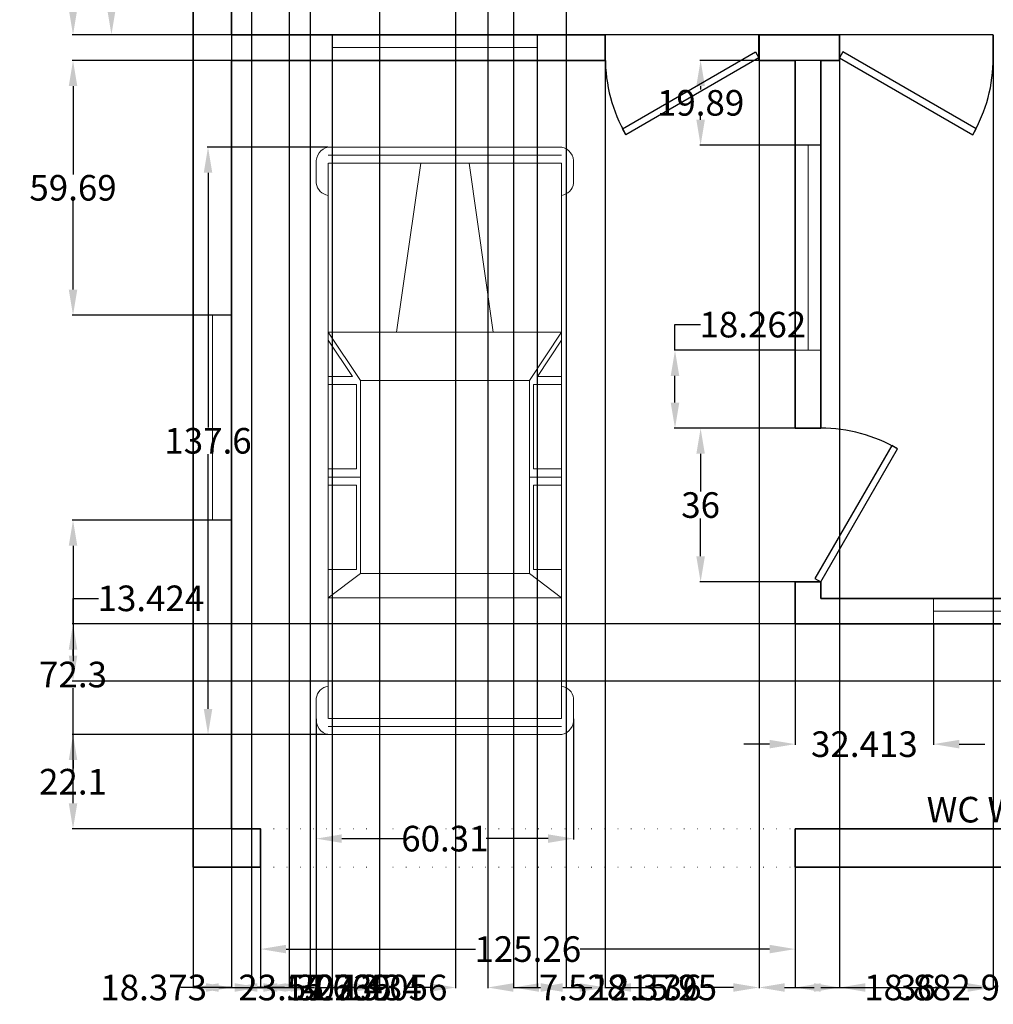
# Model space of a CAD drawing. Units: inches. Extents: x 351 to 774, y 111 to 703.
# Tile 1 of 6: x 380 to 608, y 111 to 342. Entities that reach past the tile are written whole.
import ezdxf

# ---------------------------------------------------------------- set-up
doc = ezdxf.new("R2010")
doc.units = ezdxf.units.IN
doc.header["$MEASUREMENT"] = 0
doc.linetypes.add('ACAD_ISO07W100', pattern=[3, 0, -3])
for name, color, linetype, lineweight in [('A-ANNO-DIMS', 2, 'Continuous', 18), ('A-DOOR', 3, 'Continuous', 25), ('A-EQPM-VEHC', 8, 'Continuous', 13), ('A-GLAZ', 4, 'Continuous', 18), ('A-WALL', 7, 'Continuous', 35), ('A-WALL-OVHD', 7, 'ACAD_ISO07W100', 18)]:
    doc.layers.add(name, color=color, linetype=linetype, lineweight=lineweight)
doc.styles.get("Standard").update_dxf_attribs({"font": 'arial.ttf'})
doc.dimstyles.get("Standard").update_dxf_attribs({"dimtxt": 6, "dimasz": 6, "dimexe": 0.18, "dimexo": 0.0625, "dimgap": 0.09, "dimtad": 0, "dimtih": 1, "dimtoh": 1, "dimdec": 0, "dimzin": 0, "dimdsep": 46, "dimlunit": 3, "dimtxsty": 'Standard', "dimcen": 0.09, "dimadec": 0, "dimazin": 0, "dimtfac": 1, "dimtdec": 0, "dimtofl": 0, "dimtmove": 0, "dimatfit": 3, "dimfxl": 1, "dimtolj": 1, "dimtzin": 0, "dimarcsym": 0})

# ---------------------------------------------------------------- blocks, each defined once
blk = doc.blocks.new('*U4')
for p, q in [((-40, 0), (-40, 6)), ((0, 0), (0, 6))]:
    blk.add_line(p, q)
blk.add_lwpolyline([(0, 0), (-34.64, -20), (-35.52, -18.48), (-0.88, 1.52)], close=True)
blk.add_arc((0, 0), 40, 180, 210)
blk = doc.blocks.new('*U5')
for p, q in [((0, 0), (0, 6)), ((40, 0), (40, 6))]:
    blk.add_line(p, q)
blk.add_lwpolyline([(0, 0), (34.64, -20), (35.52, -18.48), (0.88, 1.52)], close=True)
blk.add_arc((0, 0), 40, 330, 0)
blk = doc.blocks.new('*U6')
for p, q in [((0, 0), (0, -6)), ((-40, 0), (-40, -6))]:
    blk.add_line(p, q)
blk.add_lwpolyline([(0, 0), (-34.64, 20), (-35.52, 18.48), (-0.88, -1.52)], close=True)
blk.add_arc((0, 0), 40, 150, 180)
blk = doc.blocks.new('*U15')
for p, q in [((5.44, 42.31), (12.12, 42.31)), ((189.69, 42.31), (183.01, 42.31)), ((0.1, -0.41), (0.1, 38.35)), ((2.77, -0.41), (2.77, 38.31)), ((5.44, -0.41), (5.44, 38.24)), ((5.45, 38.31), (16.12, 38.31)), ((16.12, 38.31), (180.34, 38.31)), ((61.52, -0.41), (61.52, 38.31)), ((61.52, 38.31), (77.54, 27.62)), ((64.19, 38.31), (76.2, 30.29)), ((76.2, 30.29), (76.2, 38.31)), ((78.87, 38.31), (78.87, 28.96)), ((106.91, 28.96), (106.91, 38.31)), ((109.58, 27.62), (109.58, 38.31)), ((112.25, 38.31), (112.25, 28.96)), ((140.29, 28.96), (140.29, 38.31)), ((141.62, 27.62), (149.64, 38.31)), ((149.64, -0.41), (149.64, 38.31)), ((189.69, 38.31), (179.01, 38.31)), ((189.69, -0.41), (189.69, 38.24)), ((192.36, -0.41), (192.36, 38.31)), ((195.03, -0.41), (195.03, 38.35)), ((77.54, 27.62), (141.62, 27.62)), ((77.54, -0.41), (77.54, 27.62)), ((78.87, 28.96), (106.91, 28.96)), ((112.25, 28.96), (140.29, 28.96)), ((141.62, -0.41), (141.62, 27.62)), ((5.44, 7.6), (61.52, 15.61)), ((0.1, -0.42), (0.1, -39.18)), ((2.77, -0.41), (2.77, -39.13)), ((5.44, -0.42), (5.44, -39.07)), ((61.52, -0.41), (61.52, -39.13)), ((77.54, -0.41), (77.54, -28.45)), ((141.62, -0.41), (141.62, -28.45)), ((149.64, -0.41), (149.64, -39.13)), ((189.69, -0.42), (189.69, -39.07)), ((192.36, -0.41), (192.36, -39.13)), ((195.03, -0.42), (195.03, -39.18)), ((5.44, -8.42), (61.52, -16.43)), ((61.52, -39.13), (77.54, -28.45)), ((77.54, -28.45), (141.62, -28.45)), ((109.58, -28.45), (109.58, -39.13)), ((141.62, -28.45), (149.64, -39.13)), ((64.19, -39.13), (76.2, -31.12)), ((76.2, -31.12), (76.2, -39.13)), ((78.87, -39.13), (78.87, -29.79)), ((78.87, -29.79), (106.91, -29.79)), ((106.91, -29.79), (106.91, -39.13)), ((112.25, -29.79), (140.29, -29.79)), ((112.25, -39.13), (112.25, -29.79)), ((140.29, -29.79), (140.29, -39.13)), ((5.45, -39.13), (16.12, -39.13)), ((16.12, -39.13), (180.34, -39.13)), ((189.69, -39.13), (179.01, -39.13)), ((5.44, -43.14), (12.12, -43.14)), ((189.69, -43.14), (183.01, -43.14))]:
    blk.add_line(p, q)
for centre, radius, start, end in [((5.06, 37.26), 5.06, 85.6455, 168.0943), ((11.45, 37.64), 4.72, 8.1301, 81.87), ((183.68, 37.64), 4.72, 98.13, 171.8699), ((190.07, 37.26), 5.06, 11.9057, 94.3545), ((5.06, -38.09), 5.06, 191.9057, 274.3545), ((11.45, -38.46), 4.72, 278.13, 351.8699), ((183.68, -38.46), 4.72, 188.1301, 261.87), ((190.07, -38.09), 5.06, 265.6455, 348.0943)]:
    blk.add_arc(centre, radius, start, end)
blk = doc.blocks.new('WIN-48IN-6IN-WALL')
blk.add_line((3, 48), (3, 0))
blk.add_lwpolyline([(0, 48), (6, 48), (6, 0), (0, 0)], close=True)
blk = doc.blocks.new('WIN-48IN-9IN-WALL')
blk.add_line((4.5, 48), (4.5, 0))
blk.add_lwpolyline([(0, 0), (9, 0), (9, 48), (0, 48)], close=True)
blk = doc.blocks.new('*D26')
at = {"layer": 'A-ANNO-DIMS', "color": 0, "lineweight": -2, "transparency": 16777216}
for p, q in [((680.41, 152.3), (680.41, 156.92)), ((710.41, 152.3), (710.41, 156.92)), ((680.41, 156.74), (674.41, 156.74)), ((704.41, 156.74), (686.41, 156.74))]:
    blk.add_line(p, q, dxfattribs=at)
at = {"layer": 'A-ANNO-DIMS', "color": 0, "transparency": 16777216}
for points in [[(686.41, 157.74), (686.41, 155.74), (680.41, 156.74)], [(704.41, 157.74), (704.41, 155.74), (710.41, 156.74)]]:
    blk.add_solid(points, dxfattribs=at)
at = {"layer": 'Defpoints', "color": 0, "transparency": 16777216}
for p in [(680.41, 156.74), (680.41, 152.24), (710.41, 152.24)]:
    blk.add_point(p, dxfattribs=at)
at = {"layer": 'A-ANNO-DIMS', "color": 0, "transparency": 16777216, "insert": (631.89, 156.74), "char_height": 6, "attachment_point": 5}
blk.add_mtext('\\A1;WC WINDOW 30 TYP.', dxfattribs=at)
blk = doc.blocks.new('*D50')
at = {"layer": 'A-ANNO-DIMS', "color": 0, "lineweight": -2, "transparency": 16777216}
for p, q in [((421.04, 671.18), (421.04, 114.91)), ((443.48, 671.18), (443.48, 114.91)), ((427.04, 115.09), (437.48, 115.09)), ((443.48, 115.09), (449.48, 115.09))]:
    blk.add_line(p, q, dxfattribs=at)
at = {"layer": 'A-ANNO-DIMS', "color": 0, "transparency": 16777216}
for points in [[(427.04, 116.09), (427.04, 114.09), (421.04, 115.09)], [(437.48, 116.09), (437.48, 114.09), (443.48, 115.09)]]:
    blk.add_solid(points, dxfattribs=at)
at = {"layer": 'Defpoints', "color": 0, "transparency": 16777216}
for p in [(421.04, 671.24), (443.48, 671.24), (443.48, 115.09)]:
    blk.add_point(p, dxfattribs=at)
at = {"layer": 'A-ANNO-DIMS', "color": 0, "transparency": 16777216, "insert": (462.06, 115.09), "char_height": 6, "attachment_point": 5}
blk.add_mtext('\\A1;22.434', dxfattribs=at)
blk = doc.blocks.new('*D55')
at = {"layer": 'A-ANNO-DIMS', "color": 0, "lineweight": -2, "transparency": 16777216}
for p, q in [((429.98, 372.59), (392.71, 372.59)), ((392.89, 366.59), (392.89, 358.57)), ((392.89, 344.24), (392.89, 352.26)), ((429.98, 338.24), (392.71, 338.24))]:
    blk.add_line(p, q, dxfattribs=at)
at = {"layer": 'A-ANNO-DIMS', "color": 0, "transparency": 16777216}
for points in [[(391.89, 366.59), (393.89, 366.59), (392.89, 372.59)], [(391.89, 344.24), (393.89, 344.24), (392.89, 338.24)]]:
    blk.add_solid(points, dxfattribs=at)
at = {"layer": 'Defpoints', "color": 0, "transparency": 16777216}
for p in [(392.89, 372.59), (430.04, 372.59), (430.04, 338.24)]:
    blk.add_point(p, dxfattribs=at)
at = {"layer": 'A-ANNO-DIMS', "color": 0, "transparency": 16777216, "insert": (392.89, 355.41), "char_height": 6, "attachment_point": 5}
blk.add_mtext('\\A1;34.344', dxfattribs=at)
blk = doc.blocks.new('*D56')
at = {"layer": 'A-ANNO-DIMS', "color": 0, "lineweight": -2, "transparency": 16777216}
for p, q in [((429.98, 464.24), (401.71, 464.24)), ((401.89, 458.24), (401.89, 404.4)), ((401.89, 344.24), (401.89, 398.09)), ((429.98, 338.24), (401.71, 338.24))]:
    blk.add_line(p, q, dxfattribs=at)
at = {"layer": 'A-ANNO-DIMS', "color": 0, "transparency": 16777216}
for points in [[(400.89, 458.24), (402.89, 458.24), (401.89, 464.24)], [(400.89, 344.24), (402.89, 344.24), (401.89, 338.24)]]:
    blk.add_solid(points, dxfattribs=at)
at = {"layer": 'Defpoints', "color": 0, "transparency": 16777216}
for p in [(401.89, 464.24), (430.04, 464.24), (430.04, 338.24)]:
    blk.add_point(p, dxfattribs=at)
at = {"layer": 'A-ANNO-DIMS', "color": 0, "transparency": 16777216, "insert": (401.89, 401.24), "char_height": 6, "attachment_point": 5}
blk.add_mtext('\\A1;126', dxfattribs=at)
blk = doc.blocks.new('*D57')
at = {"layer": 'A-ANNO-DIMS', "color": 0, "lineweight": -2, "transparency": 16777216}
for p, q in [((429.98, 224.55), (392.71, 224.55)), ((392.89, 218.55), (392.89, 191.55)), ((392.89, 158.24), (392.89, 185.24)), ((429.98, 152.24), (392.71, 152.24))]:
    blk.add_line(p, q, dxfattribs=at)
at = {"layer": 'A-ANNO-DIMS', "color": 0, "transparency": 16777216}
for points in [[(391.89, 218.55), (393.89, 218.55), (392.89, 224.55)], [(391.89, 158.24), (393.89, 158.24), (392.89, 152.24)]]:
    blk.add_solid(points, dxfattribs=at)
at = {"layer": 'Defpoints', "color": 0, "transparency": 16777216}
for p in [(392.89, 224.55), (430.04, 224.55), (430.04, 152.24)]:
    blk.add_point(p, dxfattribs=at)
at = {"layer": 'A-ANNO-DIMS', "color": 0, "transparency": 16777216, "insert": (392.89, 188.4), "char_height": 6, "attachment_point": 5}
blk.add_mtext('\\A1;72.3', dxfattribs=at)
blk = doc.blocks.new('*D58')
at = {"layer": 'A-ANNO-DIMS', "color": 0, "lineweight": -2, "transparency": 16777216}
for p, q in [((429.98, 332.24), (392.71, 332.24)), ((392.89, 326.24), (392.89, 305.55)), ((392.89, 278.55), (392.89, 299.24)), ((429.98, 272.55), (392.71, 272.55))]:
    blk.add_line(p, q, dxfattribs=at)
at = {"layer": 'A-ANNO-DIMS', "color": 0, "transparency": 16777216}
for points in [[(391.89, 326.24), (393.89, 326.24), (392.89, 332.24)], [(391.89, 278.55), (393.89, 278.55), (392.89, 272.55)]]:
    blk.add_solid(points, dxfattribs=at)
at = {"layer": 'Defpoints', "color": 0, "transparency": 16777216}
for p in [(392.89, 332.24), (430.04, 332.24), (430.04, 272.55)]:
    blk.add_point(p, dxfattribs=at)
at = {"layer": 'A-ANNO-DIMS', "color": 0, "transparency": 16777216, "insert": (392.89, 302.4), "char_height": 6, "attachment_point": 5}
blk.add_mtext('\\A1;59.69', dxfattribs=at)
blk = doc.blocks.new('*D59')
at = {"layer": 'A-ANNO-DIMS', "color": 0, "lineweight": -2, "transparency": 16777216}
for p, q in [((436.78, 152.18), (436.78, 123.91)), ((562.04, 152.18), (562.04, 123.91)), ((442.78, 124.09), (487.15, 124.09)), ((556.04, 124.09), (511.67, 124.09))]:
    blk.add_line(p, q, dxfattribs=at)
at = {"layer": 'A-ANNO-DIMS', "color": 0, "transparency": 16777216}
for points in [[(442.78, 125.09), (442.78, 123.09), (436.78, 124.09)], [(556.04, 125.09), (556.04, 123.09), (562.04, 124.09)]]:
    blk.add_solid(points, dxfattribs=at)
at = {"layer": 'Defpoints', "color": 0, "transparency": 16777216}
for p in [(436.78, 152.24), (562.04, 152.24), (436.78, 124.09)]:
    blk.add_point(p, dxfattribs=at)
at = {"layer": 'A-ANNO-DIMS', "color": 0, "transparency": 16777216, "insert": (499.41, 124.09), "char_height": 6, "attachment_point": 5}
blk.add_mtext('\\A1;125.26', dxfattribs=at)
blk = doc.blocks.new('*D60')
at = {"layer": 'A-ANNO-DIMS', "color": 0, "lineweight": -2, "transparency": 16777216}
for p, q in [((421.04, 143.18), (421.04, 114.91)), ((436.78, 143.18), (436.78, 114.91)), ((427.04, 115.09), (430.78, 115.09)), ((436.78, 115.09), (442.78, 115.09))]:
    blk.add_line(p, q, dxfattribs=at)
at = {"layer": 'A-ANNO-DIMS', "color": 0, "transparency": 16777216}
for points in [[(427.04, 116.09), (427.04, 114.09), (421.04, 115.09)], [(430.78, 116.09), (430.78, 114.09), (436.78, 115.09)]]:
    blk.add_solid(points, dxfattribs=at)
at = {"layer": 'Defpoints', "color": 0, "transparency": 16777216}
for p in [(421.04, 143.24), (436.78, 143.24), (436.78, 115.09)]:
    blk.add_point(p, dxfattribs=at)
at = {"layer": 'A-ANNO-DIMS', "color": 0, "transparency": 16777216, "insert": (455.06, 115.09), "char_height": 6, "attachment_point": 5}
blk.add_mtext('\\A1;15.735', dxfattribs=at)
blk = doc.blocks.new('*D61')
at = {"layer": 'A-ANNO-DIMS', "color": 0, "lineweight": -2, "transparency": 16777216}
for p, q in [((562.04, 152.18), (562.04, 114.91)), ((658.04, 152.18), (658.04, 114.91)), ((568.04, 115.09), (605.66, 115.09)), ((652.04, 115.09), (614.43, 115.09))]:
    blk.add_line(p, q, dxfattribs=at)
at = {"layer": 'A-ANNO-DIMS', "color": 0, "transparency": 16777216}
for points in [[(568.04, 116.09), (568.04, 114.09), (562.04, 115.09)], [(652.04, 116.09), (652.04, 114.09), (658.04, 115.09)]]:
    blk.add_solid(points, dxfattribs=at)
at = {"layer": 'Defpoints', "color": 0, "transparency": 16777216}
for p in [(562.04, 152.24), (658.04, 152.24), (658.04, 115.09)]:
    blk.add_point(p, dxfattribs=at)
at = {"layer": 'A-ANNO-DIMS', "color": 0, "transparency": 16777216, "insert": (610.04, 115.09), "char_height": 6, "attachment_point": 5}
blk.add_mtext('\\A1;96', dxfattribs=at)
blk = doc.blocks.new('*D70')
at = {"layer": 'A-ANNO-DIMS', "color": 0, "lineweight": -2, "transparency": 16777216}
for p, q in [((430.04, 614.18), (430.04, 114.91)), ((434.71, 614.18), (434.71, 114.91)), ((424.04, 115.09), (418.04, 115.09)), ((440.71, 115.09), (446.71, 115.09))]:
    blk.add_line(p, q, dxfattribs=at)
at = {"layer": 'A-ANNO-DIMS', "color": 0, "transparency": 16777216}
for points in [[(424.04, 116.09), (424.04, 114.09), (430.04, 115.09)], [(440.71, 116.09), (440.71, 114.09), (434.71, 115.09)]]:
    blk.add_solid(points, dxfattribs=at)
at = {"layer": 'Defpoints', "color": 0, "transparency": 16777216}
for p in [(430.04, 614.24), (434.71, 614.24), (434.71, 115.09)]:
    blk.add_point(p, dxfattribs=at)
at = {"layer": 'A-ANNO-DIMS', "color": 0, "transparency": 16777216, "insert": (457.05, 115.09), "char_height": 6, "attachment_point": 5}
blk.add_mtext('\\A1;4.669', dxfattribs=at)
blk = doc.blocks.new('*D71')
at = {"layer": 'A-ANNO-DIMS', "color": 0, "lineweight": -2, "transparency": 16777216}
for p, q in [((434.71, 614.18), (434.71, 114.91)), ((464.71, 614.18), (464.71, 114.91)), ((440.71, 115.09), (445.34, 115.09)), ((458.71, 115.09), (454.09, 115.09))]:
    blk.add_line(p, q, dxfattribs=at)
at = {"layer": 'A-ANNO-DIMS', "color": 0, "transparency": 16777216}
for points in [[(440.71, 116.09), (440.71, 114.09), (434.71, 115.09)], [(458.71, 116.09), (458.71, 114.09), (464.71, 115.09)]]:
    blk.add_solid(points, dxfattribs=at)
at = {"layer": 'Defpoints', "color": 0, "transparency": 16777216}
for p in [(434.71, 614.24), (464.71, 614.24), (464.71, 115.09)]:
    blk.add_point(p, dxfattribs=at)
at = {"layer": 'A-ANNO-DIMS', "color": 0, "transparency": 16777216, "insert": (449.71, 115.09), "char_height": 6, "attachment_point": 5}
blk.add_mtext('\\A1;30', dxfattribs=at)
blk = doc.blocks.new('*D74')
at = {"layer": 'A-ANNO-DIMS', "color": 0, "lineweight": -2, "transparency": 16777216}
for p, q in [((430.043027, 338.179576), (430.043027, 114.912076)), ((453.614453, 338.179576), (453.614453, 114.912076)), ((424.043027, 115.092076), (418.043027, 115.092076)), ((459.614453, 115.092076), (465.614453, 115.092076))]:
    blk.add_line(p, q, dxfattribs=at)
at = {"layer": 'A-ANNO-DIMS', "color": 0, "transparency": 16777216}
for points in [[(424.043027, 116.092076), (424.043027, 114.092076), (430.043027, 115.092076)], [(459.614453, 116.092076), (459.614453, 114.092076), (453.614453, 115.092076)]]:
    blk.add_solid(points, dxfattribs=at)
at = {"layer": 'Defpoints', "color": 0, "transparency": 16777216}
for p in [(430.043027, 338.242076), (453.614453, 338.242076), (453.614453, 115.092076)]:
    blk.add_point(p, dxfattribs=at)
at = {"layer": 'A-ANNO-DIMS', "color": 0, "transparency": 16777216, "insert": (441.82874, 115.092076), "char_height": 6, "attachment_point": 5}
blk.add_mtext('\\A1;23.57', dxfattribs=at)
blk = doc.blocks.new('*D75')
at = {"layer": 'A-ANNO-DIMS', "color": 0, "lineweight": -2, "transparency": 16777216}
for p, q in [((501.61, 338.18), (501.61, 114.91)), ((517.57, 338.18), (517.57, 114.91)), ((507.61, 115.09), (511.57, 115.09)), ((517.57, 115.09), (523.57, 115.09))]:
    blk.add_line(p, q, dxfattribs=at)
at = {"layer": 'A-ANNO-DIMS', "color": 0, "transparency": 16777216}
for points in [[(507.61, 116.09), (507.61, 114.09), (501.61, 115.09)], [(511.57, 116.09), (511.57, 114.09), (517.57, 115.09)]]:
    blk.add_solid(points, dxfattribs=at)
at = {"layer": 'Defpoints', "color": 0, "transparency": 16777216}
for p in [(501.61, 338.24), (517.57, 338.24), (517.57, 115.09)]:
    blk.add_point(p, dxfattribs=at)
at = {"layer": 'A-ANNO-DIMS', "color": 0, "transparency": 16777216, "insert": (533.52, 115.09), "char_height": 6, "attachment_point": 5}
blk.add_mtext('\\A1;15.95', dxfattribs=at)
blk = doc.blocks.new('*D76')
at = {"layer": 'A-ANNO-DIMS', "color": 0, "lineweight": -2, "transparency": 16777216}
for p, q in [((517.57, 338.18), (517.57, 114.91)), ((553.57, 338.18), (553.57, 114.91)), ((523.57, 115.09), (531.18, 115.09)), ((547.57, 115.09), (539.95, 115.09))]:
    blk.add_line(p, q, dxfattribs=at)
at = {"layer": 'A-ANNO-DIMS', "color": 0, "transparency": 16777216}
for points in [[(523.57, 116.09), (523.57, 114.09), (517.57, 115.09)], [(547.57, 116.09), (547.57, 114.09), (553.57, 115.09)]]:
    blk.add_solid(points, dxfattribs=at)
at = {"layer": 'Defpoints', "color": 0, "transparency": 16777216}
for p in [(517.57, 338.24), (553.57, 338.24), (553.57, 115.09)]:
    blk.add_point(p, dxfattribs=at)
at = {"layer": 'A-ANNO-DIMS', "color": 0, "transparency": 16777216, "insert": (535.57, 115.09), "char_height": 6, "attachment_point": 5}
blk.add_mtext('\\A1;36', dxfattribs=at)
blk = doc.blocks.new('*D77')
at = {"layer": 'A-ANNO-DIMS', "color": 0, "lineweight": -2, "transparency": 16777216}
for p, q in [((553.57, 338.18), (553.57, 114.91)), ((572.45, 338.18), (572.45, 114.91)), ((559.57, 115.09), (566.45, 115.09)), ((572.45, 115.09), (578.45, 115.09))]:
    blk.add_line(p, q, dxfattribs=at)
at = {"layer": 'A-ANNO-DIMS', "color": 0, "transparency": 16777216}
for points in [[(559.57, 116.09), (559.57, 114.09), (553.57, 115.09)], [(566.45, 116.09), (566.45, 114.09), (572.45, 115.09)]]:
    blk.add_solid(points, dxfattribs=at)
at = {"layer": 'Defpoints', "color": 0, "transparency": 16777216}
for p in [(553.57, 338.24), (572.45, 338.24), (572.45, 115.09)]:
    blk.add_point(p, dxfattribs=at)
at = {"layer": 'A-ANNO-DIMS', "color": 0, "transparency": 16777216, "insert": (590.68, 115.09), "char_height": 6, "attachment_point": 5}
blk.add_mtext('\\A1;18.882', dxfattribs=at)
blk = doc.blocks.new('*D78')
at = {"layer": 'A-ANNO-DIMS', "color": 0, "lineweight": -2, "transparency": 16777216}
for p, q in [((572.45, 338.18), (572.45, 114.91)), ((608.45, 338.18), (608.45, 114.91)), ((578.45, 115.09), (586.06, 115.09)), ((602.45, 115.09), (594.83, 115.09))]:
    blk.add_line(p, q, dxfattribs=at)
at = {"layer": 'A-ANNO-DIMS', "color": 0, "transparency": 16777216}
for points in [[(578.45, 116.09), (578.45, 114.09), (572.45, 115.09)], [(602.45, 116.09), (602.45, 114.09), (608.45, 115.09)]]:
    blk.add_solid(points, dxfattribs=at)
at = {"layer": 'Defpoints', "color": 0, "transparency": 16777216}
for p in [(572.45, 338.24), (608.45, 338.24), (608.45, 115.09)]:
    blk.add_point(p, dxfattribs=at)
at = {"layer": 'A-ANNO-DIMS', "color": 0, "transparency": 16777216, "insert": (590.45, 115.09), "char_height": 6, "attachment_point": 5}
blk.add_mtext('\\A1;36', dxfattribs=at)
blk = doc.blocks.new('*D82')
at = {"layer": 'A-ANNO-DIMS', "color": 0, "lineweight": -2, "transparency": 16777216}
for p, q in [((567.98, 246.09), (539.71, 246.09)), ((539.89, 240.09), (539.89, 231.25)), ((539.89, 216.09), (539.89, 224.93)), ((567.98, 210.09), (539.71, 210.09))]:
    blk.add_line(p, q, dxfattribs=at)
at = {"layer": 'A-ANNO-DIMS', "color": 0, "transparency": 16777216}
for points in [[(538.89, 240.09), (540.89, 240.09), (539.89, 246.09)], [(538.89, 216.09), (540.89, 216.09), (539.89, 210.09)]]:
    blk.add_solid(points, dxfattribs=at)
at = {"layer": 'Defpoints', "color": 0, "transparency": 16777216}
for p in [(539.89, 246.09), (568.04, 246.09), (568.04, 210.09)]:
    blk.add_point(p, dxfattribs=at)
at = {"layer": 'A-ANNO-DIMS', "color": 0, "transparency": 16777216, "insert": (539.89, 228.09), "char_height": 6, "attachment_point": 5}
blk.add_mtext('\\A1;36', dxfattribs=at)
blk = doc.blocks.new('*D83')
at = {"layer": 'A-ANNO-DIMS', "color": 0, "lineweight": -2, "transparency": 16777216}
for p, q in [((533.89, 264.35), (533.89, 270.35)), ((533.89, 270.35), (539.89, 270.35)), ((561.98, 264.35), (533.71, 264.35)), ((533.89, 252.09), (533.89, 258.35)), ((561.98, 246.09), (533.71, 246.09))]:
    blk.add_line(p, q, dxfattribs=at)
at = {"layer": 'A-ANNO-DIMS', "color": 0, "transparency": 16777216}
for points in [[(532.89, 258.35), (534.89, 258.35), (533.89, 264.35)], [(532.89, 252.09), (534.89, 252.09), (533.89, 246.09)]]:
    blk.add_solid(points, dxfattribs=at)
at = {"layer": 'Defpoints', "color": 0, "transparency": 16777216}
for p in [(533.89, 264.35), (562.04, 264.35), (562.04, 246.09)]:
    blk.add_point(p, dxfattribs=at)
at = {"layer": 'A-ANNO-DIMS', "color": 0, "transparency": 16777216, "insert": (552.12, 270.35), "char_height": 6, "attachment_point": 5}
blk.add_mtext('\\A1;18.262', dxfattribs=at)
blk = doc.blocks.new('*D84')
at = {"layer": 'A-ANNO-DIMS', "color": 0, "lineweight": -2, "transparency": 16777216}
for p, q in [((567.98, 332.24), (539.71, 332.24)), ((539.89, 326.24), (539.89, 325.45)), ((539.89, 318.35), (539.89, 319.14)), ((567.98, 312.35), (539.71, 312.35))]:
    blk.add_line(p, q, dxfattribs=at)
at = {"layer": 'A-ANNO-DIMS', "color": 0, "transparency": 16777216}
for points in [[(538.89, 326.24), (540.89, 326.24), (539.89, 332.24)], [(538.89, 318.35), (540.89, 318.35), (539.89, 312.35)]]:
    blk.add_solid(points, dxfattribs=at)
at = {"layer": 'Defpoints', "color": 0, "transparency": 16777216}
for p in [(539.89, 332.24), (568.04, 332.24), (568.04, 312.35)]:
    blk.add_point(p, dxfattribs=at)
at = {"layer": 'A-ANNO-DIMS', "color": 0, "transparency": 16777216, "insert": (539.89, 322.3), "char_height": 6, "attachment_point": 5}
blk.add_mtext('\\A1;19.89', dxfattribs=at)
blk = doc.blocks.new('*D85')
at = {"layer": 'A-ANNO-DIMS', "color": 0, "lineweight": -2, "transparency": 16777216}
for p, q in [((562.043027, 200.179576), (562.043027, 171.912076)), ((594.456315, 200.179576), (594.456315, 171.912076)), ((556.043027, 172.092076), (550.043027, 172.092076)), ((600.456315, 172.092076), (606.456315, 172.092076))]:
    blk.add_line(p, q, dxfattribs=at)
at = {"layer": 'A-ANNO-DIMS', "color": 0, "transparency": 16777216}
for points in [[(556.043027, 173.092076), (556.043027, 171.092076), (562.043027, 172.092076)], [(600.456315, 173.092076), (600.456315, 171.092076), (594.456315, 172.092076)]]:
    blk.add_solid(points, dxfattribs=at)
at = {"layer": 'Defpoints', "color": 0, "transparency": 16777216}
for p in [(562.043027, 200.242076), (594.456315, 200.242076), (562.043027, 172.092076)]:
    blk.add_point(p, dxfattribs=at)
at = {"layer": 'A-ANNO-DIMS', "color": 0, "transparency": 16777216, "insert": (578.249671, 172.092076), "char_height": 6, "attachment_point": 5}
blk.add_mtext('\\A1;32.413', dxfattribs=at)
blk = doc.blocks.new('*D91')
at = {"layer": 'A-ANNO-DIMS', "color": 0, "lineweight": -2, "transparency": 16777216}
for p, q in [((496.04, 614.18), (496.04, 114.91)), ((508.41, 614.18), (508.41, 114.91)), ((502.04, 115.09), (502.41, 115.09)), ((508.41, 115.09), (514.41, 115.09))]:
    blk.add_line(p, q, dxfattribs=at)
at = {"layer": 'A-ANNO-DIMS', "color": 0, "transparency": 16777216}
for points in [[(502.04, 116.09), (502.04, 114.09), (496.04, 115.09)], [(502.41, 116.09), (502.41, 114.09), (508.41, 115.09)]]:
    blk.add_solid(points, dxfattribs=at)
at = {"layer": 'Defpoints', "color": 0, "transparency": 16777216}
for p in [(496.04, 614.24), (508.41, 614.24), (508.41, 115.09)]:
    blk.add_point(p, dxfattribs=at)
at = {"layer": 'A-ANNO-DIMS', "color": 0, "transparency": 16777216, "insert": (526.65, 115.09), "char_height": 6, "attachment_point": 5}
blk.add_mtext('\\A1;12.372', dxfattribs=at)
blk = doc.blocks.new('*D92')
at = {"layer": 'A-ANNO-DIMS', "color": 0, "lineweight": -2, "transparency": 16777216}
for p, q in [((449.83, 178.05), (449.83, 149.78)), ((510.15, 178.05), (510.15, 149.78)), ((455.83, 149.96), (470.34, 149.96)), ((504.15, 149.96), (489.64, 149.96))]:
    blk.add_line(p, q, dxfattribs=at)
at = {"layer": 'A-ANNO-DIMS', "color": 0, "transparency": 16777216}
for points in [[(455.83, 150.96), (455.83, 148.96), (449.83, 149.96)], [(504.15, 150.96), (504.15, 148.96), (510.15, 149.96)]]:
    blk.add_solid(points, dxfattribs=at)
at = {"layer": 'Defpoints', "color": 0, "transparency": 16777216}
for p in [(449.83, 178.11), (510.15, 178.11), (449.83, 149.96)]:
    blk.add_point(p, dxfattribs=at)
at = {"layer": 'A-ANNO-DIMS', "color": 0, "transparency": 16777216, "insert": (479.99, 149.96), "char_height": 6, "attachment_point": 5}
blk.add_mtext('\\A1;60.31', dxfattribs=at)
blk = doc.blocks.new('*D93')
at = {"layer": 'A-ANNO-DIMS', "color": 0, "lineweight": -2, "transparency": 16777216}
for p, q in [((452.6, 311.93), (424.33, 311.93)), ((424.51, 305.93), (424.51, 246.29)), ((424.51, 180.34), (424.51, 239.98)), ((452.6, 174.34), (424.33, 174.34))]:
    blk.add_line(p, q, dxfattribs=at)
at = {"layer": 'A-ANNO-DIMS', "color": 0, "transparency": 16777216}
for points in [[(423.51, 305.93), (425.51, 305.93), (424.51, 311.93)], [(423.51, 180.34), (425.51, 180.34), (424.51, 174.34)]]:
    blk.add_solid(points, dxfattribs=at)
at = {"layer": 'Defpoints', "color": 0, "transparency": 16777216}
for p in [(424.51, 311.93), (452.66, 311.93), (452.66, 174.34)]:
    blk.add_point(p, dxfattribs=at)
at = {"layer": 'A-ANNO-DIMS', "color": 0, "transparency": 16777216, "insert": (424.51, 243.14), "char_height": 6, "attachment_point": 5}
blk.add_mtext('\\A1;137.6', dxfattribs=at)
blk = doc.blocks.new('*D97')
at = {"layer": 'A-ANNO-DIMS', "color": 0, "lineweight": -2, "transparency": 16777216}
for p, q in [((602.76, 359.47), (392.71, 359.47)), ((392.89, 353.47), (392.89, 352.01)), ((392.89, 344.24), (392.89, 345.7)), ((608.38, 338.24), (392.71, 338.24))]:
    blk.add_line(p, q, dxfattribs=at)
at = {"layer": 'A-ANNO-DIMS', "color": 0, "transparency": 16777216}
for points in [[(391.89, 353.47), (393.89, 353.47), (392.89, 359.47)], [(391.89, 344.24), (393.89, 344.24), (392.89, 338.24)]]:
    blk.add_solid(points, dxfattribs=at)
at = {"layer": 'Defpoints', "color": 0, "transparency": 16777216}
for p in [(602.82, 359.47), (392.89, 338.24), (608.45, 338.24)]:
    blk.add_point(p, dxfattribs=at)
at = {"layer": 'A-ANNO-DIMS', "color": 0, "transparency": 16777216, "insert": (392.89, 348.86), "char_height": 6, "attachment_point": 5}
blk.add_mtext('\\A1;21.233', dxfattribs=at)
blk = doc.blocks.new('*D99')
at = {"layer": 'A-ANNO-DIMS', "color": 0, "lineweight": -2, "transparency": 16777216}
for p, q in [((482.51, 629.76), (482.51, 114.91)), ((490.04, 614.18), (490.04, 114.91)), ((476.51, 115.09), (470.51, 115.09)), ((496.04, 115.09), (502.04, 115.09))]:
    blk.add_line(p, q, dxfattribs=at)
at = {"layer": 'A-ANNO-DIMS', "color": 0, "transparency": 16777216}
for points in [[(476.51, 116.09), (476.51, 114.09), (482.51, 115.09)], [(496.04, 116.09), (496.04, 114.09), (490.04, 115.09)]]:
    blk.add_solid(points, dxfattribs=at)
at = {"layer": 'Defpoints', "color": 0, "transparency": 16777216}
for p in [(482.51, 629.82), (490.04, 614.24), (490.04, 115.09)]:
    blk.add_point(p, dxfattribs=at)
at = {"layer": 'A-ANNO-DIMS', "color": 0, "transparency": 16777216, "insert": (512.24, 115.09), "char_height": 6, "attachment_point": 5}
blk.add_mtext('\\A1;7.528', dxfattribs=at)
blk = doc.blocks.new('*D100')
at = {"layer": 'A-ANNO-DIMS', "color": 0, "lineweight": -2, "transparency": 16777216}
for p, q in [((430.04, 662.18), (430.04, 114.91)), ((448.42, 661.61), (448.42, 114.91)), ((430.04, 115.09), (424.04, 115.09)), ((442.42, 115.09), (436.04, 115.09))]:
    blk.add_line(p, q, dxfattribs=at)
at = {"layer": 'A-ANNO-DIMS', "color": 0, "transparency": 16777216}
for points in [[(436.04, 116.09), (436.04, 114.09), (430.04, 115.09)], [(442.42, 116.09), (442.42, 114.09), (448.42, 115.09)]]:
    blk.add_solid(points, dxfattribs=at)
at = {"layer": 'Defpoints', "color": 0, "transparency": 16777216}
for p in [(430.04, 662.24), (448.42, 661.68), (430.04, 115.09)]:
    blk.add_point(p, dxfattribs=at)
at = {"layer": 'A-ANNO-DIMS', "color": 0, "transparency": 16777216, "insert": (411.78, 115.09), "char_height": 6, "attachment_point": 5}
blk.add_mtext('\\A1;18.373', dxfattribs=at)
blk = doc.blocks.new('*D102')
at = {"layer": 'A-ANNO-DIMS', "color": 0, "lineweight": -2, "transparency": 16777216}
for p, q in [((392.89, 200.24), (392.89, 206.24)), ((392.89, 206.24), (398.89, 206.24)), ((663.98, 200.24), (392.71, 200.24)), ((392.89, 192.82), (392.89, 194.24)), ((670.45, 186.82), (392.71, 186.82))]:
    blk.add_line(p, q, dxfattribs=at)
at = {"layer": 'A-ANNO-DIMS', "color": 0, "transparency": 16777216}
for points in [[(391.89, 194.24), (393.89, 194.24), (392.89, 200.24)], [(391.89, 192.82), (393.89, 192.82), (392.89, 186.82)]]:
    blk.add_solid(points, dxfattribs=at)
at = {"layer": 'Defpoints', "color": 0, "transparency": 16777216}
for p in [(392.89, 200.24), (664.04, 200.24), (670.51, 186.82)]:
    blk.add_point(p, dxfattribs=at)
at = {"layer": 'A-ANNO-DIMS', "color": 0, "transparency": 16777216, "insert": (411.14, 206.24), "char_height": 6, "attachment_point": 5}
blk.add_mtext('\\A1;13.424', dxfattribs=at)
blk = doc.blocks.new('*D106')
at = {"layer": 'A-ANNO-DIMS', "color": 0, "lineweight": -2, "transparency": 16777216}
for p, q in [((449.83, 178.05), (449.83, 114.91)), ((436.78, 152.18), (436.78, 114.91)), ((442.78, 115.09), (443.83, 115.09)), ((449.83, 115.09), (455.83, 115.09))]:
    blk.add_line(p, q, dxfattribs=at)
at = {"layer": 'A-ANNO-DIMS', "color": 0, "transparency": 16777216}
for points in [[(442.78, 116.09), (442.78, 114.09), (436.78, 115.09)], [(443.83, 116.09), (443.83, 114.09), (449.83, 115.09)]]:
    blk.add_solid(points, dxfattribs=at)
at = {"layer": 'Defpoints', "color": 0, "transparency": 16777216}
for p in [(449.83, 178.11), (436.78, 152.24), (449.83, 115.09)]:
    blk.add_point(p, dxfattribs=at)
at = {"layer": 'A-ANNO-DIMS', "color": 0, "transparency": 16777216, "insert": (468.09, 115.09), "char_height": 6, "attachment_point": 5}
blk.add_mtext('\\A1;13.056', dxfattribs=at)
blk = doc.blocks.new('*D107')
at = {"layer": 'A-ANNO-DIMS', "color": 0, "lineweight": -2, "transparency": 16777216}
for p, q in [((452.6, 174.34), (392.71, 174.34)), ((392.89, 168.34), (392.89, 166.39)), ((392.89, 158.24), (392.89, 160.19)), ((436.72, 152.24), (392.71, 152.24))]:
    blk.add_line(p, q, dxfattribs=at)
at = {"layer": 'A-ANNO-DIMS', "color": 0, "transparency": 16777216}
for points in [[(391.89, 168.34), (393.89, 168.34), (392.89, 174.34)], [(391.89, 158.24), (393.89, 158.24), (392.89, 152.24)]]:
    blk.add_solid(points, dxfattribs=at)
at = {"layer": 'Defpoints', "color": 0, "transparency": 16777216}
for p in [(392.89, 174.34), (452.66, 174.34), (436.78, 152.24)]:
    blk.add_point(p, dxfattribs=at)
at = {"layer": 'A-ANNO-DIMS', "color": 0, "transparency": 16777216, "insert": (392.89, 163.29), "char_height": 6, "attachment_point": 5}
blk.add_mtext('\\A1;22.1', dxfattribs=at)

msp = doc.modelspace()

# ---------------------------------------------------------------- linework, layer by layer
at = {"layer": 'A-WALL'}
for p, q in [((430.043, 338.2421), (430.043, 464.2421)), ((517.5653, 338.2421), (430.043, 338.2421)), ((517.5653, 332.2421), (517.5653, 338.2421)), ((553.5653, 332.2421), (553.5653, 338.2421)), ((572.4474, 338.2421), (553.5653, 338.2421)), ((572.4474, 332.2421), (572.4474, 338.2421)), ((430.043, 152.2421), (430.043, 332.2421)), ((517.5653, 332.2421), (430.043, 332.2421)), ((562.043, 332.2421), (553.5653, 332.2421)), ((562.043, 246.0897), (562.043, 332.2421)), ((568.043, 246.0897), (568.043, 332.2421)), ((572.4474, 332.2421), (568.043, 332.2421)), ((562.043, 246.0897), (568.043, 246.0897)), ((562.043, 200.2421), (562.043, 210.0897)), ((562.043, 210.0897), (568.043, 210.0897)), ((568.043, 206.2421), (568.043, 210.0897)), ((691.5107, 206.2421), (568.043, 206.2421)), ((658.043, 200.2421), (562.043, 200.2421)), ((436.7781, 152.2421), (430.043, 152.2421)), ((436.7781, 152.2421), (436.7781, 143.2421)), ((562.043, 152.2421), (562.043, 143.2421)), ((658.043, 152.2421), (562.043, 152.2421))]:
    msp.add_line(p, q, dxfattribs=at)
msp.add_lwpolyline([(436.7781, 143.2421), (421.043, 143.2421), (421.043, 671.2421), (733.043, 671.2421), (733.043, 143.2421), (562.043, 143.2421)], dxfattribs=at)
at = {"layer": 'A-WALL-OVHD'}
for p, q in [((436.7781, 152.2421), (562.043, 152.2421)), ((436.7781, 143.2421), (562.043, 143.2421))]:
    msp.add_line(p, q, dxfattribs=at)

# ---------------------------------------------------------------- block references
at = {"layer": 'A-DOOR', "xscale": 0.8999999999999985, "yscale": 0.8999999999999985, "zscale": 0.8999999999999985}
for name, p in [('*U4', (553.5653, 332.8421)), ('*U5', (572.4474, 332.8421))]:
    msp.add_blockref(name, p, dxfattribs=at)
at = {"layer": 'A-DOOR', "xscale": 0.8999999999999985, "yscale": 0.8999999999999985, "zscale": 0.8999999999999985, "rotation": 269.9999999999995}
msp.add_blockref('*U6', (568.043, 210.0897), dxfattribs=at)
at = {"layer": 'A-EQPM-VEHC', "xscale": 0.705869788754301, "yscale": 0.705869788754301, "zscale": 0.705869788754301, "rotation": 270}
msp.add_blockref('*U15', (480.2827, 312.0066), dxfattribs=at)
at = {"layer": 'A-GLAZ'}
for p, rotation in [((501.6145, 332.2421), 89.99999999999976), ((642.4563, 200.2421), 90.00000000000006)]:
    msp.add_blockref('WIN-48IN-6IN-WALL', p, dxfattribs=dict(at, rotation=rotation))
for name, p in [('WIN-48IN-6IN-WALL', (562.043, 264.3517)), ('WIN-48IN-9IN-WALL', (421.043, 224.5483))]:
    msp.add_blockref(name, p, dxfattribs=at)

# ---------------------------------------------------------------- dimensions: what is measured, and where the dimension line sits
at = {"layer": 'A-ANNO-DIMS'}
for base, p1, p2, override, picture, middle in [((443.4772, 115.0921), (421.043, 671.2421), (443.4772, 671.2421), {"dimdec": 3, "dimlfac": 1, "dimrnd": 0, "dimzin": 0, "dimdsep": 46, "dimlunit": 2}, '*D50', (462.0604, 115.0921)), ((430.043, 115.0921), (448.416, 661.6763), (430.043, 662.2421), {"dimdec": 3, "dimlfac": 1, "dimrnd": 0, "dimzin": 0, "dimdsep": 46, "dimlunit": 2}, '*D100', (411.7811, 115.0921)), ((490.043, 115.0921), (482.5147, 629.8184), (490.043, 614.2421), {"dimdec": 3, "dimlfac": 1, "dimrnd": 0, "dimzin": 0, "dimdsep": 46, "dimlunit": 2}, '*D99', (512.2381, 115.0921)), ((434.7119, 115.0921), (430.043, 614.2421), (434.7119, 614.2421), {"dimdec": 3, "dimlfac": 1, "dimrnd": 0, "dimzin": 0, "dimdsep": 46, "dimlunit": 2}, '*D70', (457.0522, 115.0921)), ((464.7119, 115.0921), (434.7119, 614.2421), (464.7119, 614.2421), {"dimdec": 0, "dimlfac": 1, "dimrnd": 0, "dimzin": 0, "dimdsep": 46, "dimlunit": 2}, '*D71', (449.7119, 115.0921)), ((508.4146, 115.0921), (496.043, 614.2421), (508.4146, 614.2421), {"dimdec": 3, "dimlfac": 1, "dimrnd": 0, "dimzin": 0, "dimdsep": 46, "dimlunit": 2}, '*D91', (526.6458, 115.0921)), ((453.6145, 115.0921), (430.043, 338.2421), (453.6145, 338.2421), {"dimdec": 2, "dimlfac": 1, "dimrnd": 0, "dimzin": 0, "dimdsep": 46, "dimlunit": 2}, '*D74', (441.8287, 115.0921)), ((517.5653, 115.0921), (501.6145, 338.2421), (517.5653, 338.2421), {"dimdec": 2, "dimlfac": 1, "dimrnd": 0, "dimzin": 0, "dimdsep": 46, "dimlunit": 2}, '*D75', (533.5189, 115.0921)), ((553.5653, 115.0921), (517.5653, 338.2421), (553.5653, 338.2421), {"dimdec": 0, "dimlfac": 1, "dimrnd": 0, "dimzin": 0, "dimdsep": 46, "dimlunit": 2}, '*D76', (535.5653, 115.0921)), ((572.4474, 115.0921), (553.5653, 338.2421), (572.4474, 338.2421), {"dimdec": 3, "dimlfac": 1, "dimrnd": 0, "dimzin": 0, "dimdsep": 46, "dimlunit": 2}, '*D77', (590.6786, 115.0921)), ((608.4474, 115.0921), (572.4474, 338.2421), (608.4474, 338.2421), {"dimdec": 0, "dimlfac": 1, "dimrnd": 0, "dimzin": 0, "dimdsep": 46, "dimlunit": 2}, '*D78', (590.4474, 115.0921)), ((449.8337, 115.0921), (436.7781, 152.2421), (449.8337, 178.1111), {"dimdec": 3, "dimlfac": 1, "dimrnd": 0, "dimzin": 0, "dimdsep": 46, "dimlunit": 2}, '*D106', (468.0935, 115.0921)), ((658.043, 115.0921), (562.043, 152.2421), (658.043, 152.2421), {"dimdec": 0, "dimlfac": 1, "dimrnd": 0, "dimzin": 0, "dimdsep": 46, "dimlunit": 2}, '*D61', (610.043, 115.0921)), ((436.7781, 115.0921), (421.043, 143.2421), (436.7781, 143.2421), {"dimdec": 3, "dimlfac": 1, "dimrnd": 0, "dimzin": 0, "dimdsep": 46, "dimlunit": 2}, '*D60', (455.0625, 115.0921))]:
    dim = msp.add_linear_dim(base=base, p1=p1, p2=p2, dimstyle='Standard', override=override, dxfattribs=at)
    dim.commit()
    dim.dimension.update_dxf_attribs({"geometry": picture, "text_midpoint": middle})
for base, p1, p2, angle, override, picture, middle in [((401.893, 464.2421), (430.043, 338.2421), (430.043, 464.2421), 90, {"dimdec": 0, "dimlfac": 1, "dimrnd": 0, "dimzin": 0, "dimdsep": 46, "dimlunit": 2}, '*D56', (401.893, 401.2421)), ((392.89303, 372.58657), (430.04303, 338.24208), (430.04303, 372.58657), 90, {"dimdec": 3, "dimlfac": 1, "dimrnd": 0, "dimzin": 0, "dimdsep": 46, "dimlunit": 2}, '*D55', (392.89303, 355.41432)), ((392.89303, 338.24208), (602.82353, 359.47464), (608.44737, 338.24208), 90, {"dimdec": 3, "dimlfac": 1, "dimrnd": 0, "dimzin": 0, "dimdsep": 46, "dimlunit": 2}, '*D97', (392.89303, 348.85836)), ((392.893, 332.2421), (430.043, 272.5483), (430.043, 332.2421), 90, {"dimdec": 2, "dimlfac": 1, "dimrnd": 0, "dimzin": 0, "dimdsep": 46, "dimlunit": 2}, '*D58', (392.893, 302.3952)), ((539.893, 332.2421), (568.043, 312.3517), (568.043, 332.2421), 90, {"dimdec": 2, "dimlfac": 1, "dimrnd": 0, "dimzin": 0, "dimdsep": 46, "dimlunit": 2}, '*D84', (539.893, 322.2969)), ((424.511, 311.9344), (452.661, 174.3415), (452.661, 311.9344), 90, {"dimdec": 1, "dimlfac": 1, "dimrnd": 0, "dimzin": 0, "dimdsep": 46, "dimlunit": 2}, '*D93', (424.511, 243.138)), ((533.893, 264.3517), (562.043, 246.0897), (562.043, 264.3517), 90, {"dimdec": 3, "dimlfac": 1, "dimrnd": 0, "dimzin": 0, "dimdsep": 46, "dimlunit": 2}, '*D83', (552.1242, 270.3517)), ((539.893, 246.0897), (568.043, 210.0897), (568.043, 246.0897), 90, {"dimdec": 0, "dimlfac": 1, "dimrnd": 0, "dimzin": 0, "dimdsep": 46, "dimlunit": 2}, '*D82', (539.893, 228.0897)), ((392.893, 224.5483), (430.043, 152.2421), (430.043, 224.5483), 90, {"dimdec": 1, "dimlfac": 1, "dimrnd": 0, "dimzin": 0, "dimdsep": 46, "dimlunit": 2}, '*D57', (392.893, 188.3952)), ((392.893, 200.2421), (670.5147, 186.8184), (664.043, 200.2421), 90, {"dimdec": 3, "dimlfac": 1, "dimrnd": 0, "dimzin": 0, "dimdsep": 46, "dimlunit": 2}, '*D102', (411.1426, 206.2421)), ((562.043, 172.0921), (594.4563, 200.2421), (562.043, 200.2421), 180, {"dimdec": 3, "dimlfac": 1, "dimrnd": 0, "dimzin": 0, "dimdsep": 46, "dimlunit": 2}, '*D85', (578.2497, 172.0921)), ((449.8337, 149.9611), (510.1484, 178.1111), (449.8337, 178.1111), 180, {"dimdec": 2, "dimlfac": 1, "dimrnd": 0, "dimzin": 0, "dimdsep": 46, "dimlunit": 2}, '*D92', (479.991, 149.9611)), ((392.893, 174.3415), (436.7781, 152.2421), (452.661, 174.3415), 90, {"dimdec": 1, "dimlfac": 1, "dimrnd": 0, "dimzin": 0, "dimdsep": 46, "dimlunit": 2}, '*D107', (392.893, 163.2918)), ((436.7781, 124.0921), (562.043, 152.2421), (436.7781, 152.2421), 180, {"dimdec": 2, "dimlfac": 1, "dimrnd": 0, "dimzin": 0, "dimdsep": 46, "dimlunit": 2}, '*D59', (499.4105, 124.0921))]:
    dim = msp.add_linear_dim(base=base, p1=p1, p2=p2, angle=angle, dimstyle='Standard', override=override, dxfattribs=at)
    dim.commit()
    dim.dimension.update_dxf_attribs({"geometry": picture, "text_midpoint": middle})
dim = msp.add_linear_dim(base=(680.4102, 156.7421), p1=(710.4102, 152.2421), p2=(680.4102, 152.2421), angle=180, text='WC WINDOW <> TYP.', dimstyle='Standard', override={"dimdec": 0, "dimlfac": 1, "dimrnd": 0, "dimzin": 0, "dimdsep": 46, "dimlunit": 2}, dxfattribs=at)
dim.commit()
dim.dimension.update_dxf_attribs({"geometry": '*D26', "text_midpoint": (631.8946, 156.7421)})

doc.saveas('drawing.dxf')
